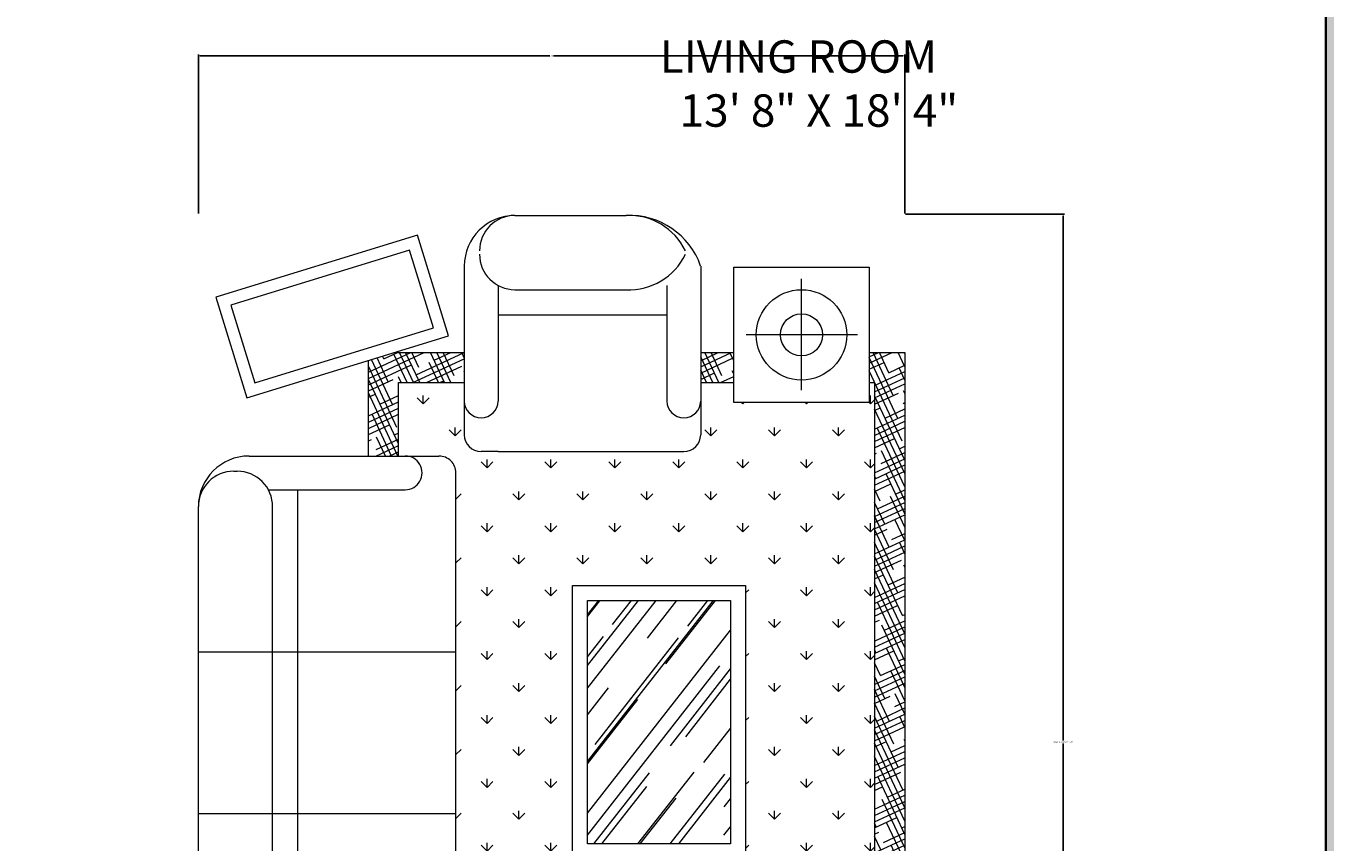
# Model space of a CAD drawing. Units: inches. Extents: x 2701 to 6846, y 811 to 2447.
# Tile 13 of 20: x 2926 to 3086, y 1130 to 1231. Entities that reach past the tile are written whole.
import ezdxf

# ---------------------------------------------------------------- set-up
doc = ezdxf.new("R2010")
doc.units = ezdxf.units.IN
for name, color, linetype, lineweight in [('A-ANNO-DIMS', 2, 'Continuous', 18), ('A-AREA-IDEN', 7, 'Continuous', 18), ('A-FURN', 8, 'Continuous', 13), ('A-WALL', 7, 'Continuous', 35)]:
    doc.layers.add(name, color=color, linetype=linetype, lineweight=lineweight)
doc.layers.add('A-WALL-PATT', color=18, linetype='Continuous', lineweight=13, true_color=0x000000)
doc.styles.get("Standard").update_dxf_attribs({"font": 'arial.ttf'})
doc.dimstyles.get("Standard").update_dxf_attribs({"dimtxt": 0.18, "dimasz": 0.18, "dimexe": 0.18, "dimexo": 0.0625, "dimgap": 0.09, "dimtad": 0, "dimtih": 1, "dimtoh": 1, "dimdec": 4, "dimzin": 0, "dimdsep": 46, "dimtxsty": 'Standard', "dimcen": 0.09, "dimadec": 0, "dimazin": 0, "dimtfac": 1, "dimtdec": 4, "dimtofl": 0, "dimtmove": 0, "dimatfit": 3, "dimfxl": 1, "dimtolj": 1, "dimtzin": 0, "dimarcsym": 0})

# ---------------------------------------------------------------- blocks, each defined once
blk = doc.blocks.new('A$C0782773B')
for p, q in [((1027.2, 2344.2), (2528, 2344.2)), ((1508.8, 2344.2), (1508.8, 1489.7)), ((2046.4, 2344.2), (2046.4, 1489.7)), ((3223.5, 2286.1), (2888.9, 2183.3)), ((3429.1, 1617), (3223.5, 2286.1)), ((909.6, 2226.6), (909.6, 2215.4)), ((2645.6, 2226.6), (2645.6, 2215.4)), ((3197, 2236.1), (2938.9, 2156.8)), ((3379.1, 1643.5), (3197, 2236.1)), ((859.2, 2176.2), (859.2, 1545.7)), ((2696, 2176.2), (2696, 1545.7)), ((2888.9, 2183.3), (3094.6, 1514.2)), ((2938.9, 2156.8), (3121.1, 1564.2)), ((971.2, 2111.9), (971.2, 1657.7)), ((1027.2, 2097.8), (2528, 2097.8)), ((2584, 2111.9), (2584, 1657.7)), ((971.2, 2013.8), (2584, 2013.8)), ((622.9, 1770.7), (643.4, 1780.2)), ((622.9, 1750), (687.8, 1780.2)), ((622.9, 1729.3), (732.1, 1780.2)), ((622.9, 1380.2), (622.9, 1780.2)), ((622.9, 1780.2), (859.2, 1780.2)), ((627.3, 1710.7), (776.5, 1780.2)), ((636.3, 1780.2), (637.5, 1777.5)), ((657, 1780.2), (686.2, 1717.5)), ((677.6, 1780.2), (724.3, 1680.2)), ((698.3, 1780.2), (745, 1680.2)), ((703.2, 1725.4), (820.8, 1780.2)), ((719, 1780.2), (765.7, 1680.2)), ((779.1, 1740.1), (859.2, 1777.4)), ((781.1, 1780.2), (788.2, 1765)), ((801.8, 1780.2), (836.9, 1705)), ((822.5, 1780.2), (859.2, 1701.5)), ((843.2, 1780.2), (859.2, 1745.8)), ((2696, 1682.3), (2906.1, 1780.2)), ((2696, 1780.2), (3012.8, 1780.2)), ((2736, 1680.2), (2950.4, 1780.2)), ((2746.5, 1780.2), (2751.2, 1770.1)), ((2767.2, 1780.2), (2799.9, 1710.1)), ((2787.9, 1780.2), (2834.5, 1680.2)), ((2790.8, 1685.1), (2994.8, 1780.2)), ((2808.5, 1780.2), (2855.2, 1680.2)), ((2829.2, 1780.2), (2875.9, 1680.2)), ((2866.7, 1699.8), (3016.1, 1769.5)), ((2891.3, 1780.2), (2901.9, 1757.6)), ((2912, 1780.2), (2950.5, 1697.6)), ((2932.7, 1780.2), (2999.2, 1637.5)), ((2953.4, 1780.2), (3039.7, 1595.1)), ((2974, 1780.2), (3039.7, 1639.5)), ((754.2, 1749.2), (786.3, 1680.2)), ((855, 1754.8), (859.2, 1756.8)), ((2696, 1703), (2835, 1767.8)), ((2696, 1755.4), (2731, 1680.2)), ((2696, 1723.7), (2759.1, 1753.1)), ((2717.2, 1754.3), (2751.7, 1680.2)), ((2867.9, 1741.8), (2896.6, 1680.2)), ((2942.6, 1714.5), (3021.7, 1751.4)), ((3018.5, 1729.2), (3027.2, 1733.3)), ((3018.5, 1729.2), (3039.7, 1683.9)), ((622.9, 1720.3), (722.9, 1505.8)), ((622.9, 1646.6), (719.1, 1691.4)), ((652.2, 1701.6), (722.9, 1550.2)), ((739.5, 1680.2), (795, 1706.1)), ((783.9, 1680.2), (859.2, 1715.4)), ((802.9, 1689.1), (807, 1680.2)), ((828.2, 1680.2), (859.2, 1694.7)), ((2696, 1711), (2710.4, 1680.2)), ((2765.9, 1694.2), (2772.4, 1680.2)), ((2939.7, 1651.1), (3034.4, 1695.3)), ((3039.7, 1692.8), (3039.7, 1461.7)), ((622.9, 1667.2), (643.2, 1676.7)), ((622.9, 1675.9), (681.6, 1549.8)), ((622.9, 1625.9), (722.9, 1672.5)), ((622.9, 1605.2), (722.9, 1651.8)), ((700.9, 1641.6), (722.9, 1594.5)), ((722.9, 1340.4), (722.9, 1680.2)), ((722.9, 1680.2), (859.2, 1680.2)), ((2696, 1680.2), (2939.7, 1680.2)), ((2916.6, 1681.7), (2917.2, 1680.2)), ((2939.7, 1671.8), (2958.5, 1680.6)), ((2939.7, 1680.2), (2939.7, 1461.7)), ((2939.7, 1630.4), (3039.7, 1677.1)), ((2939.7, 1609.7), (3039.7, 1656.4)), ((3121.1, 1564.2), (3379.1, 1643.5)), ((622.9, 1631.5), (633, 1609.9)), ((674.9, 1608.7), (722.9, 1631.1)), ((747.4, 1598.5), (767.3, 1618.4)), ((747.4, 1598.5), (775.6, 1598.5)), ((747.4, 1598.5), (767.3, 1578.6)), ((2868.8, 1598.5), (2888.7, 1618.4)), ((2868.8, 1598.5), (2896.9, 1598.5)), ((2868.8, 1598.5), (2888.7, 1578.6)), ((2939.7, 1632.1), (3019.1, 1461.7)), ((2965.3, 1621.7), (3039.7, 1462)), ((2990.2, 1612.6), (3039.7, 1635.7)), ((3094.6, 1514.2), (3429.1, 1617)), ((622.9, 1543.1), (690.7, 1574.7)), ((622.9, 1522.4), (722.9, 1569.1)), ((2939.7, 1587.7), (2994.7, 1469.9)), ((2939.7, 1547.7), (3006, 1578.6)), ((2939.7, 1527), (3039.7, 1573.6)), ((3013.9, 1561.6), (3039.7, 1506.4)), ((622.9, 1501.7), (722.9, 1548.4)), ((622.9, 1542.8), (715.9, 1343.2)), ((646.5, 1492.1), (722.9, 1527.7)), ((647.7, 1534), (722.9, 1372.7)), ((853.5, 1492.5), (871.6, 1510.6)), ((2762.7, 1492.5), (2782.6, 1512.3)), ((2939.7, 1506.3), (3039.7, 1552.9)), ((2939.7, 1543.4), (2946, 1529.9)), ((2961.8, 1495.9), (3039.7, 1532.2)), ((3037.7, 1510.6), (3039.7, 1511.5)), ((395.3, 1470.7), (915.7, 1263.8)), ((622.9, 1498.4), (677.1, 1382.2)), ((696.4, 1473.9), (722.9, 1417.1)), ((722.4, 1506.8), (722.9, 1507)), ((853.5, 1492.5), (881.6, 1492.5)), ((853.5, 1492.5), (873.4, 1472.6)), ((915.2, 1489.7), (2640, 1489.7)), ((1068.4, 1489.7), (1085.5, 1472.6)), ((1280.5, 1489.7), (1297.7, 1472.6)), ((1492.7, 1489.7), (1509.8, 1472.6)), ((1704.8, 1489.7), (1721.9, 1472.6)), ((1916.9, 1489.7), (1934.1, 1472.6)), ((2129.1, 1489.7), (2146.2, 1472.6)), ((2341.2, 1489.7), (2358.3, 1472.6)), ((2553.3, 1489.7), (2570.5, 1472.6)), ((2762.7, 1492.5), (2790.8, 1492.5)), ((2762.7, 1492.5), (2782.6, 1472.6)), ((3021.6, 1461.7), (3039.7, 1470.2)), ((622.9, 1419), (722.9, 1465.6)), ((622.9, 1439.7), (662.4, 1458.1)), ((622.9, 1454.1), (628.4, 1442.2)), ((622.9, 1398.3), (722.9, 1444.9)), ((625.9, 1379), (722.9, 1424.2)), ((3326.7, 1461.7), (2766.7, 1461.7)), ((2977.2, 1461.7), (2977.7, 1461.9)), ((694.1, 1390.1), (722.9, 1403.5)), ((747.4, 1386.4), (767.3, 1406.3)), ((747.4, 1386.4), (775.6, 1386.4)), ((747.4, 1386.4), (767.3, 1366.5)), ((959.6, 1386.4), (979.5, 1406.3)), ((959.6, 1386.4), (987.7, 1386.4)), ((959.6, 1386.4), (979.5, 1366.5)), ((1171.7, 1386.4), (1191.6, 1406.3)), ((1171.7, 1386.4), (1199.8, 1386.4)), ((1171.7, 1386.4), (1191.6, 1366.5)), ((1383.8, 1386.4), (1403.7, 1406.3)), ((1383.8, 1386.4), (1412, 1386.4)), ((1383.8, 1386.4), (1403.7, 1366.5)), ((1596, 1386.4), (1615.9, 1406.3)), ((1596, 1386.4), (1624.1, 1386.4)), ((1596, 1386.4), (1615.9, 1366.5)), ((1808.1, 1386.4), (1828, 1406.3)), ((1808.1, 1386.4), (1836.2, 1386.4)), ((1808.1, 1386.4), (1828, 1366.5)), ((2020.2, 1386.4), (2040.1, 1406.3)), ((2020.2, 1386.4), (2048.4, 1386.4)), ((2020.2, 1386.4), (2040.1, 1366.5)), ((2232.4, 1386.4), (2252.3, 1406.3)), ((2232.4, 1386.4), (2260.5, 1386.4)), ((2232.4, 1386.4), (2252.3, 1366.5)), ((2444.5, 1386.4), (2464.4, 1406.3)), ((2444.5, 1386.4), (2472.6, 1386.4)), ((2444.5, 1386.4), (2464.4, 1366.5)), ((2656.6, 1386.4), (2676.5, 1406.3)), ((2656.6, 1386.4), (2684.8, 1386.4)), ((2656.6, 1386.4), (2676.5, 1366.5)), ((2710.7, 1349.7), (2710.7, 1405.7)), ((413.6, 1342.9), (770.2, 1201.1)), ((697.7, 1350.4), (709.9, 1356.1)), ((721.7, 1340.9), (722.9, 1341.5)), ((2710.7, 1349.7), (2710.7, 733.3)), ((3262.5, 1349.7), (2878.7, 1349.7)), ((3164.3, 1349.7), (3164.3, 789.3)), ((11.5, 960), (148, 1303.4)), ((297.8, 785.9), (504.9, 1306.6)), ((859.4, 1286.2), (873.4, 1300.2)), ((1065.6, 1280.3), (1085.5, 1300.2)), ((1277.8, 1280.3), (1297.7, 1300.2)), ((1489.9, 1280.3), (1509.8, 1300.2)), ((1702, 1280.3), (1721.9, 1300.2)), ((1914.2, 1280.3), (1934.1, 1300.2)), ((2126.3, 1280.3), (2146.2, 1300.2)), ((2338.4, 1280.3), (2358.3, 1300.2)), ((2550.6, 1280.3), (2570.5, 1300.2)), ((874.1, 1280.3), (881.6, 1280.3)), ((1065.6, 1280.3), (1093.8, 1280.3)), ((1065.6, 1280.3), (1085.5, 1260.4)), ((1277.8, 1280.3), (1305.9, 1280.3)), ((1277.8, 1280.3), (1297.7, 1260.4)), ((1489.9, 1280.3), (1518, 1280.3)), ((1489.9, 1280.3), (1509.8, 1260.4)), ((1702, 1280.3), (1730.2, 1280.3)), ((1702, 1280.3), (1721.9, 1260.4)), ((1914.2, 1280.3), (1942.3, 1280.3)), ((1914.2, 1280.3), (1934.1, 1260.4)), ((2126.3, 1280.3), (2154.4, 1280.3)), ((2126.3, 1280.3), (2146.2, 1260.4)), ((2338.4, 1280.3), (2366.6, 1280.3)), ((2338.4, 1280.3), (2358.3, 1260.4)), ((2550.6, 1280.3), (2578.7, 1280.3)), ((2550.6, 1280.3), (2570.5, 1260.4)), ((3248.3, 1293.7), (3248.3, 924.1)), ((3494.7, 1293.7), (3494.7, 924.1)), ((240.4, 868.9), (377, 1212.4)), ((719.3, 618.3), (947, 1191)), ((959.6, 1174.3), (979.5, 1194.1)), ((959.6, 1174.3), (987.7, 1174.3)), ((959.6, 1174.3), (979.5, 1154.4)), ((1171.7, 1174.3), (1191.6, 1194.1)), ((1171.7, 1174.3), (1199.8, 1174.3)), ((1171.7, 1174.3), (1191.6, 1154.4)), ((1383.8, 1174.3), (1403.7, 1194.1)), ((1383.8, 1174.3), (1412, 1174.3)), ((1383.8, 1174.3), (1403.7, 1154.4)), ((1596, 1174.3), (1615.9, 1194.1)), ((1596, 1174.3), (1624.1, 1174.3)), ((1596, 1174.3), (1615.9, 1154.4)), ((1808.1, 1174.3), (1828, 1194.1)), ((1808.1, 1174.3), (1836.2, 1174.3)), ((1808.1, 1174.3), (1828, 1154.4)), ((2020.2, 1174.3), (2040.1, 1194.1)), ((2020.2, 1174.3), (2048.4, 1174.3)), ((2020.2, 1174.3), (2040.1, 1154.4)), ((2232.4, 1174.3), (2252.3, 1194.1)), ((2232.4, 1174.3), (2260.5, 1174.3)), ((2232.4, 1174.3), (2252.3, 1154.4)), ((2444.5, 1174.3), (2464.4, 1194.1)), ((2444.5, 1174.3), (2472.6, 1174.3)), ((2444.5, 1174.3), (2464.4, 1154.4)), ((2656.6, 1174.3), (2676.5, 1194.1)), ((2656.6, 1174.3), (2684.8, 1174.3)), ((2656.6, 1174.3), (2676.5, 1154.4)), ((1065.6, 1068.2), (1085.5, 1088.1)), ((1277.8, 1068.2), (1297.7, 1088.1)), ((1358.2, 528.2), (1358.2, 1102.6)), ((1358.2, 1102.6), (2266.7, 1102.6)), ((2266.7, 1102.6), (2266.7, 528.2)), ((2338.4, 1068.2), (2358.3, 1088.1)), ((2550.6, 1068.2), (2570.5, 1088.1)), ((1065.6, 1068.2), (1093.8, 1068.2)), ((1065.6, 1068.2), (1085.5, 1048.3)), ((1277.8, 1068.2), (1305.9, 1068.2)), ((1277.8, 1068.2), (1297.7, 1048.3)), ((1408.2, 578.2), (1408.2, 1052.6)), ((1408.2, 1052.6), (2216.7, 1052.6)), ((1437.7, 1052.6), (1999.3, 613.9)), ((1510.8, 1052.6), (2118.1, 578.2)), ((1674, 1052.6), (1887.9, 885.5)), ((1681.3, 1052.6), (2216.7, 634.3)), ((1837.3, 1052.6), (1926.1, 983.2)), ((1925, 1052.6), (2216.7, 824.7)), ((2000.5, 1052.6), (2216.7, 883.7)), ((2029.7, 1052.6), (2097.2, 999.9)), ((2163.7, 1052.6), (2215.4, 1012.3)), ((2168.6, 1052.6), (2216.7, 1015)), ((2216.7, 1052.6), (2216.7, 578.2)), ((2338.4, 1068.2), (2366.6, 1068.2)), ((2338.4, 1068.2), (2358.3, 1048.3)), ((2550.6, 1068.2), (2578.7, 1068.2)), ((2550.6, 1068.2), (2570.5, 1048.3)), ((1408.2, 1031.9), (1644.7, 847.1)), ((1408.2, 1005.3), (1598.7, 856.4)), ((1738, 1027.4), (2092.6, 750.4)), ((959.6, 962.1), (979.5, 982)), ((959.6, 962.1), (987.7, 962.1)), ((959.6, 962.1), (979.5, 942.2)), ((1171.7, 962.1), (1191.6, 982)), ((1171.7, 962.1), (1199.8, 962.1)), ((1171.7, 962.1), (1191.6, 942.2)), ((2136.2, 969.5), (2216.7, 906.5)), ((2444.5, 962.1), (2464.4, 982)), ((2444.5, 962.1), (2472.6, 962.1)), ((2444.5, 962.1), (2464.4, 942.2)), ((2656.6, 962.1), (2676.5, 982)), ((2656.6, 962.1), (2684.8, 962.1)), ((2656.6, 962.1), (2676.5, 942.2)), ((853.5, 856.1), (873.4, 876)), ((1065.6, 856.1), (1085.5, 876)), ((1277.8, 856.1), (1297.7, 876)), ((1408.2, 885.3), (1646.9, 698.8)), ((1408.2, 877.7), (1560.4, 758.8)), ((2338.4, 856.1), (2358.3, 876)), ((2550.6, 856.1), (2570.5, 876)), ((206.6, 822.1), (563.2, 680.3)), ((853.5, 856.1), (881.6, 856.1)), ((853.5, 856.1), (873.4, 836.2)), ((1065.6, 856.1), (1093.8, 856.1)), ((1065.6, 856.1), (1085.5, 836.2)), ((1277.8, 856.1), (1305.9, 856.1)), ((1277.8, 856.1), (1297.7, 836.2)), ((2091.6, 853.9), (2216.7, 756.2)), ((2338.4, 856.1), (2366.6, 856.1)), ((2338.4, 856.1), (2358.3, 836.2)), ((2550.6, 856.1), (2578.7, 856.1)), ((2550.6, 856.1), (2570.5, 836.2)), ((1408.2, 778.7), (1640.1, 597.6)), ((1733.4, 777.9), (1989, 578.2)), ((2006.1, 793.2), (2216.7, 628.6)), ((3262.5, 789.3), (2878.7, 789.3)), ((105.5, 741.8), (625.9, 534.9)), ((771.7, 750), (775.6, 750)), ((959.6, 750), (979.5, 769.9)), ((959.6, 750), (987.7, 750)), ((959.6, 750), (979.5, 730.1)), ((1171.7, 750), (1191.6, 769.9)), ((1171.7, 750), (1199.8, 750)), ((1171.7, 750), (1191.6, 730.1)), ((1408.2, 750.2), (1628.4, 578.2)), ((2444.5, 750), (2464.4, 769.9)), ((2444.5, 750), (2472.6, 750)), ((2444.5, 750), (2464.4, 730.1)), ((2656.6, 750), (2676.5, 769.9)), ((2656.6, 750), (2684.8, 750)), ((2656.6, 750), (2676.5, 730.1)), ((764.8, 732.7), (767.3, 730.1)), ((1764.2, 727.1), (1954.8, 578.2)), ((2131.6, 719.9), (2216.7, 653.4)), ((853.5, 643.9), (873.4, 663.8)), ((1065.6, 643.9), (1085.5, 663.8)), ((1277.8, 643.9), (1297.7, 663.8)), ((1678.6, 666.4), (1791.6, 578.2)), ((2338.4, 643.9), (2358.3, 663.8)), ((2550.6, 643.9), (2570.5, 663.8)), ((2762.7, 643.9), (2782.6, 663.8)), ((3326.7, 677.3), (2766.7, 677.3)), ((2939.7, 658.1), (2981, 677.3)), ((2939.7, 637.4), (3025.4, 677.3)), ((2939.7, 677.3), (2939.7, 567.7)), ((2939.7, 616.7), (3039.7, 663.3)), ((2950.4, 677.3), (2971.8, 631.6)), ((2971.1, 677.3), (3020.4, 571.6)), ((2991.8, 677.3), (3039.7, 574.7)), ((3012.5, 677.3), (3039.7, 619.1)), ((3039.7, 677.3), (3039.7, 567.7)), ((719.3, 618.3), (698.6, 566.2)), ((722.9, 100), (722.9, 627.2)), ((853.5, 643.9), (881.6, 643.9)), ((853.5, 643.9), (873.4, 624)), ((1065.6, 643.9), (1093.8, 643.9)), ((1065.6, 643.9), (1085.5, 624)), ((1277.8, 643.9), (1305.9, 643.9)), ((1277.8, 643.9), (1297.7, 624)), ((2338.4, 643.9), (2366.6, 643.9)), ((2338.4, 643.9), (2358.3, 624)), ((2550.6, 643.9), (2578.7, 643.9)), ((2550.6, 643.9), (2570.5, 624)), ((2762.7, 643.9), (2790.8, 643.9)), ((2762.7, 643.9), (2782.6, 624)), ((2939.7, 611.7), (2960.2, 567.7)), ((2962.7, 606.7), (3039.7, 642.6)), ((3038.6, 621.4), (3039.7, 621.9)), ((697.8, 564.3), (722.9, 576)), ((701.9, 574.6), (722.9, 529.8)), ((722.1, 575.7), (722.9, 574.1)), ((2216.7, 578.2), (1408.2, 578.2)), ((1436.7, 600.4), (1465.1, 578.2)), ((1530.9, 599.1), (1557.7, 578.2)), ((2873.3, 567.7), (3323.3, 567.7)), ((2873.3, 117.7), (2873.3, 567.7)), ((2967.7, 567.7), (2978.5, 572.7)), ((3012, 567.7), (3039.7, 580.6)), ((3323.3, 567.7), (3323.3, 117.7)), ((622.9, 508.7), (722.9, 555.3)), ((622.9, 0), (622.9, 536.1)), ((622.9, 488), (722.9, 534.6)), ((622.9, 529.4), (630.9, 533.1)), ((622.9, 522.4), (722.9, 307.9)), ((676.8, 539.8), (702.9, 483.9)), ((691.3, 553.2), (722.9, 485.4)), ((747.4, 537.9), (767.3, 557.8)), ((747.4, 537.9), (775.6, 537.9)), ((747.4, 537.9), (767.3, 518)), ((959.6, 537.9), (979.5, 557.8)), ((959.6, 537.9), (987.7, 537.9)), ((959.6, 537.9), (979.5, 518)), ((1171.7, 537.9), (1191.6, 557.8)), ((1171.7, 537.9), (1199.8, 537.9)), ((1171.7, 537.9), (1191.6, 518)), ((2266.7, 528.2), (1358.2, 528.2)), ((1393.5, 528.2), (1403.7, 518)), ((1605.7, 528.2), (1615.9, 518)), ((1817.8, 528.2), (1828, 518)), ((2029.9, 528.2), (2040.1, 518)), ((2242.1, 528.2), (2252.3, 518)), ((2444.5, 537.9), (2464.4, 557.8)), ((2444.5, 537.9), (2472.6, 537.9)), ((2444.5, 537.9), (2464.4, 518)), ((2656.6, 537.9), (2676.5, 557.8)), ((2656.6, 537.9), (2684.8, 537.9)), ((2656.6, 537.9), (2676.5, 518)), ((2868.8, 537.9), (2873.3, 542.4)), ((2868.8, 537.9), (2873.3, 537.9)), ((2868.8, 537.9), (2873.3, 533.3)), ((3098.3, 156.5), (3098.3, 526.4)), ((622.9, 478), (698.3, 316.3)), ((694.9, 500.9), (722.9, 513.9)), ((622.9, 425.9), (710.8, 466.9)), ((622.9, 446.6), (634.9, 452.2)), ((622.9, 405.3), (722.9, 451.9)), ((622.9, 433.6), (649.6, 376.3)), ((668.9, 468.1), (722.9, 352.3)), ((853.5, 431.8), (873.4, 451.7)), ((853.5, 431.8), (881.6, 431.8)), ((853.5, 431.8), (873.4, 411.9)), ((1065.6, 431.8), (1085.5, 451.7)), ((1065.6, 431.8), (1093.8, 431.8)), ((1065.6, 431.8), (1085.5, 411.9)), ((1277.8, 431.8), (1297.7, 451.7)), ((1277.8, 431.8), (1305.9, 431.8)), ((1277.8, 431.8), (1297.7, 411.9)), ((1489.9, 431.8), (1509.8, 451.7)), ((1489.9, 431.8), (1518, 431.8)), ((1489.9, 431.8), (1509.8, 411.9)), ((1702, 431.8), (1721.9, 451.7)), ((1702, 431.8), (1730.2, 431.8)), ((1702, 431.8), (1721.9, 411.9)), ((1914.2, 431.8), (1934.1, 451.7)), ((1914.2, 431.8), (1942.3, 431.8)), ((1914.2, 431.8), (1934.1, 411.9)), ((2126.3, 431.8), (2146.2, 451.7)), ((2126.3, 431.8), (2154.4, 431.8)), ((2126.3, 431.8), (2146.2, 411.9)), ((2338.4, 431.8), (2358.3, 451.7)), ((2338.4, 431.8), (2366.6, 431.8)), ((2338.4, 431.8), (2358.3, 411.9)), ((2550.6, 431.8), (2570.5, 451.7)), ((2550.6, 431.8), (2578.7, 431.8)), ((2550.6, 431.8), (2570.5, 411.9)), ((2762.7, 431.8), (2782.6, 451.7)), ((2762.7, 431.8), (2790.8, 431.8)), ((2762.7, 431.8), (2782.6, 411.9)), ((622.9, 384.6), (722.9, 431.2)), ((666.6, 384.3), (722.9, 410.5)), ((717.6, 408), (722.9, 396.7)), ((622.9, 322.5), (682.4, 350.3)), ((622.9, 301.8), (722.9, 348.4)), ((747.4, 325.7), (767.3, 345.6)), ((959.6, 325.7), (979.5, 345.6)), ((1171.7, 325.7), (1191.6, 345.6)), ((1383.8, 325.7), (1403.7, 345.6)), ((1596, 325.7), (1615.9, 345.6)), ((1808.1, 325.7), (1828, 345.6)), ((2020.2, 325.7), (2040.1, 345.6)), ((2232.4, 325.7), (2252.3, 345.6)), ((2444.5, 325.7), (2464.4, 345.6)), ((2656.6, 325.7), (2676.5, 345.6)), ((622.9, 344.9), (722.9, 130.5)), ((622.9, 281.1), (722.9, 327.8)), ((638.2, 267.6), (722.9, 307.1)), ((747.4, 325.7), (775.6, 325.7)), ((747.4, 325.7), (767.3, 305.8)), ((959.6, 325.7), (987.7, 325.7)), ((959.6, 325.7), (979.5, 305.8)), ((1171.7, 325.7), (1199.8, 325.7)), ((1171.7, 325.7), (1191.6, 305.8)), ((1383.8, 325.7), (1412, 325.7)), ((1383.8, 325.7), (1403.7, 305.8)), ((1596, 325.7), (1624.1, 325.7)), ((1596, 325.7), (1615.9, 305.8)), ((1808.1, 325.7), (1836.2, 325.7)), ((1808.1, 325.7), (1828, 305.8)), ((2020.2, 325.7), (2048.4, 325.7)), ((2020.2, 325.7), (2040.1, 305.8)), ((2232.4, 325.7), (2260.5, 325.7)), ((2232.4, 325.7), (2252.3, 305.8)), ((2444.5, 325.7), (2472.6, 325.7)), ((2444.5, 325.7), (2464.4, 305.8)), ((2656.6, 325.7), (2684.8, 325.7)), ((2656.6, 325.7), (2676.5, 305.8)), ((2868.8, 325.7), (2873.3, 330.3)), ((2868.8, 325.7), (2873.3, 325.7)), ((2868.8, 325.7), (2873.3, 321.2)), ((2914.5, 342.7), (3284.1, 342.7)), ((622.9, 300.5), (693.7, 148.6)), ((664.3, 300.4), (722.9, 174.8)), ((714.1, 282.3), (722.9, 286.4)), ((622.9, 256.2), (645, 208.7)), ((622.9, 198.4), (722.9, 245)), ((622.9, 219.1), (654.1, 233.6)), ((622.9, 177.7), (722.9, 224.3)), ((713, 240.4), (722.9, 219.2)), ((853.5, 219.7), (873.4, 239.6)), ((853.5, 219.7), (881.6, 219.7)), ((853.5, 219.7), (873.4, 199.8)), ((1065.6, 219.7), (1085.5, 239.6)), ((1065.6, 219.7), (1093.8, 219.7)), ((1065.6, 219.7), (1085.5, 199.8)), ((1277.8, 219.7), (1297.7, 239.6)), ((1277.8, 219.7), (1305.9, 219.7)), ((1277.8, 219.7), (1297.7, 199.8)), ((1489.9, 219.7), (1509.8, 239.6)), ((1489.9, 219.7), (1518, 219.7)), ((1489.9, 219.7), (1509.8, 199.8)), ((1702, 219.7), (1721.9, 239.6)), ((1702, 219.7), (1730.2, 219.7)), ((1702, 219.7), (1721.9, 199.8)), ((1914.2, 219.7), (1934.1, 239.6)), ((1914.2, 219.7), (1942.3, 219.7)), ((1914.2, 219.7), (1934.1, 199.8)), ((2126.3, 219.7), (2146.2, 239.6)), ((2126.3, 219.7), (2154.4, 219.7)), ((2126.3, 219.7), (2146.2, 199.8)), ((2338.4, 219.7), (2358.3, 239.6)), ((2338.4, 219.7), (2366.6, 219.7)), ((2338.4, 219.7), (2358.3, 199.8)), ((2550.6, 219.7), (2570.5, 239.6)), ((2550.6, 219.7), (2578.7, 219.7)), ((2550.6, 219.7), (2570.5, 199.8)), ((2762.7, 219.7), (2782.6, 239.6)), ((2762.7, 219.7), (2790.8, 219.7)), ((2762.7, 219.7), (2782.6, 199.8)), ((622.9, 157), (722.9, 203.6)), ((685.8, 165.6), (722.9, 182.9)), ((622.9, 167.4), (700.9, 0)), ((622.9, 94.9), (701.6, 131.7)), ((659.7, 132.8), (721.6, 0)), ((747.4, 113.6), (767.3, 133.5)), ((959.6, 113.6), (979.5, 133.5)), ((1171.7, 113.6), (1191.6, 133.5)), ((1383.8, 113.6), (1403.7, 133.5)), ((1596, 113.6), (1615.9, 133.5)), ((1808.1, 113.6), (1828, 133.5)), ((2020.2, 113.6), (2040.1, 133.5)), ((2232.4, 113.6), (2252.3, 133.5)), ((2444.5, 113.6), (2464.4, 133.5)), ((2656.6, 113.6), (2676.5, 133.5)), ((622.9, 123.1), (680.3, 0)), ((622.9, 74.2), (722.9, 120.9)), ((622.9, 115.6), (625.7, 116.9)), ((622.9, 53.5), (722.9, 100.2)), ((657.4, 49), (766.8, 100)), ((2939.7, 100), (722.9, 100)), ((733.3, 63.7), (811.2, 100)), ((737.1, 100), (742.4, 88.6)), ((747.4, 113.6), (775.6, 113.6)), ((747.4, 113.6), (761, 100)), ((757.8, 100), (791.1, 28.5)), ((778.4, 100), (825.1, 0)), ((799.1, 100), (845.8, 0)), ((809.2, 78.4), (855.6, 100)), ((819.8, 100), (866.5, 0)), ((863, 0), (1052.8, 88.5)), ((881.9, 100), (893, 76.1)), ((885.1, 93.1), (899.9, 100)), ((902.6, 100), (941.7, 16)), ((907.3, 0), (1121.8, 100)), ((923.3, 100), (969.9, 0)), ((943.9, 100), (990.6, 0)), ((951.7, 0), (1166.1, 100)), ((959.6, 113.6), (987.7, 113.6)), ((959.6, 113.6), (973.2, 100)), ((964.6, 100), (1011.3, 0)), ((1008.6, 5.8), (1210.5, 100)), ((1026.7, 100), (1043.7, 63.6)), ((1047.4, 100), (1092.4, 3.5)), ((1068.1, 100), (1114.7, 0)), ((1084.4, 20.5), (1254.9, 100)), ((1088.8, 100), (1135.4, 0)), ((1111.7, 95.3), (1156.1, 0)), ((1160.3, 35.2), (1299.2, 100)), ((1171.5, 100), (1194.3, 51.1)), ((1171.7, 113.6), (1199.8, 113.6)), ((1171.7, 113.6), (1185.3, 100)), ((1192.2, 100), (1238.8, 0)), ((1212.9, 100), (1259.5, 0)), ((1233.6, 100), (1280.2, 0)), ((1236.2, 49.9), (1343.6, 100)), ((1295.7, 100), (1296.3, 98.6)), ((1312.1, 64.6), (1388, 100)), ((1316.3, 100), (1345, 38.6)), ((1337, 100), (1383.7, 0)), ((1357.7, 100), (1404.3, 0)), ((1378.4, 100), (1425, 0)), ((1383.8, 113.6), (1412, 113.6)), ((1383.8, 113.6), (1397.4, 100)), ((1388, 79.3), (1432.3, 100)), ((1439.7, 0), (1631.6, 89.5)), ((1440.5, 100), (1446.9, 86.1)), ((1461.2, 100), (1495.6, 26.1)), ((1463.9, 94), (1476.7, 100)), ((1481.8, 100), (1528.5, 0)), ((1484.1, 0), (1698.5, 100)), ((1502.5, 100), (1549.2, 0)), ((1523.2, 100), (1569.9, 0)), ((1528.5, 0), (1742.9, 100)), ((1585.3, 100), (1597.6, 73.6)), ((1587.4, 6.8), (1787.3, 100)), ((1596, 113.6), (1624.1, 113.6)), ((1596, 113.6), (1609.6, 100)), ((1606, 100), (1646.3, 13.6)), ((1626.7, 100), (1673.3, 0)), ((1647.4, 100), (1694, 0)), ((1663.3, 21.5), (1831.6, 100)), ((1668, 100), (1714.7, 0)), ((1730.1, 100), (1748.2, 61.1)), ((1739.2, 36.2), (1876, 100)), ((1750.8, 100), (1796.9, 1.1)), ((1771.5, 100), (1818.1, 0)), ((1792.2, 100), (1838.8, 0)), ((1808.1, 113.6), (1836.2, 113.6)), ((1808.1, 113.6), (1821.7, 100)), ((1815.1, 50.9), (1920.4, 100)), ((1816.2, 92.8), (1859.5, 0)), ((1874.9, 100), (1898.9, 48.6)), ((1891, 65.6), (1964.7, 100)), ((1895.6, 100), (1942.2, 0)), ((1916.3, 100), (1962.9, 0)), ((1937, 100), (1983.6, 0)), ((1966.9, 80.3), (2009.1, 100)), ((1999.1, 100), (2000.8, 96.2)), ((2016.5, 0), (2210.4, 90.4)), ((2019.7, 100), (2049.5, 36.1)), ((2020.2, 113.6), (2048.4, 113.6)), ((2020.2, 113.6), (2033.8, 100)), ((2040.4, 100), (2087.1, 0)), ((2042.8, 95), (2053.5, 100)), ((2060.8, 0), (2275.3, 100)), ((2061.1, 100), (2107.8, 0)), ((2081.8, 100), (2128.4, 0)), ((2105.2, 0), (2319.7, 100)), ((2143.9, 100), (2151.5, 83.6)), ((2164.6, 100), (2200.2, 23.6)), ((2166.2, 7.8), (2364, 100)), ((2185.2, 100), (2231.9, 0)), ((2205.9, 100), (2252.6, 0)), ((2226.6, 100), (2273.3, 0)), ((2232.4, 113.6), (2260.5, 113.6)), ((2232.4, 113.6), (2246, 100)), ((2242.1, 22.5), (2408.4, 100)), ((2288.7, 100), (2302.1, 71.1)), ((2309.4, 100), (2350.8, 11.1)), ((2318, 37.2), (2452.8, 100)), ((2330.1, 100), (2376.7, 0)), ((2350.8, 100), (2397.4, 0)), ((2371.4, 100), (2418.1, 0)), ((2393.9, 51.9), (2497.1, 100)), ((2433.5, 100), (2452.8, 58.6)), ((2444.5, 113.6), (2472.6, 113.6)), ((2444.5, 113.6), (2458.1, 100)), ((2454.2, 100), (2500.8, 0)), ((2469.8, 66.6), (2541.5, 100)), ((2474.9, 100), (2521.5, 0)), ((2495.6, 100), (2542.2, 0)), ((2520.8, 90.3), (2562.9, 0)), ((2545.7, 81.3), (2585.9, 100)), ((2578.3, 100), (2603.4, 46.1)), ((2593.2, 0), (2789.2, 91.4)), ((2599, 100), (2645.6, 0)), ((2619.7, 100), (2666.3, 0)), ((2621.6, 96), (2630.2, 100)), ((2637.6, 0), (2852.1, 100)), ((2640.4, 100), (2687, 0)), ((2656.6, 113.6), (2684.8, 113.6)), ((2656.6, 113.6), (2670.2, 100)), ((2682, 0), (2896.4, 100)), ((2702.5, 100), (2705.4, 93.7)), ((2723.1, 100), (2754.1, 33.6)), ((2743.8, 100), (2790.5, 0)), ((2745, 8.7), (2978.7, 117.7)), ((2764.5, 100), (2811.2, 0)), ((2785.2, 100), (2831.8, 0)), ((2820.9, 23.4), (3023, 117.7)), ((2847.3, 100), (2856.1, 81.2)), ((2868, 100), (2904.7, 21.1)), ((2868.8, 113.6), (2873.3, 118.1)), ((2868.8, 113.6), (2896.9, 113.6)), ((2868.8, 113.6), (2882.4, 100)), ((3323.3, 117.7), (2873.3, 117.7)), ((2888.7, 100), (2935.3, 0)), ((2896.8, 38.1), (3039.7, 104.7)), ((2909.3, 100), (2956, 0)), ((2930, 100), (2976.7, 0)), ((2939.7, 117.7), (2939.7, 100)), ((2983.9, 117.7), (3006.7, 68.7)), ((3004.5, 117.7), (3039.7, 42.3)), ((3025.2, 117.7), (3039.7, 86.7)), ((3039.7, 117.7), (3039.7, 0)), ((622.9, 78.7), (640.4, 41)), ((708.4, 72.7), (742.3, 0)), ((729.9, 0), (825.1, 44.4)), ((774.2, 0), (901, 59.1)), ((818.6, 0), (976.9, 73.8)), ((859, 60.2), (887.1, 0)), ((1009.7, 47.7), (1032, 0)), ((1262.3, 82.8), (1300.9, 0)), ((1306.6, 0), (1403.9, 45.4)), ((1351, 0), (1479.8, 60.1)), ((1395.4, 0), (1555.7, 74.8)), ((1413, 70.3), (1445.7, 0)), ((1563.6, 57.8), (1590.5, 0)), ((1714.3, 45.3), (1735.4, 0)), ((1883.4, 0), (1982.7, 46.3)), ((1927.7, 0), (2058.6, 61)), ((1966.9, 80.3), (2004.3, 0)), ((1972.1, 0), (2134.5, 75.7)), ((2117.5, 67.8), (2149.1, 0)), ((2268.2, 55.3), (2293.9, 0)), ((2460.1, 0), (2561.5, 47.3)), ((2504.5, 0), (2637.4, 62)), ((2548.9, 0), (2713.3, 76.7)), ((2671.4, 77.8), (2707.7, 0)), ((2822.1, 65.3), (2852.5, 0)), ((2972.7, 52.8), (3039.7, 84.1)), ((2972.7, 52.8), (2997.3, 0)), ((641.1, 0), (673.3, 15)), ((685.5, 0), (749.2, 29.7)), ((757.1, 12.7), (763, 0)), ((907.7, 0.2), (907.8, 0)), ((1160.3, 35.2), (1176.8, 0)), ((1173.5, 0), (1176.2, 1.2)), ((1217.9, 0), (1252.1, 15.9)), ((1262.3, 0), (1328, 30.7)), ((1311, 22.7), (1321.6, 0)), ((1461.6, 10.2), (1466.4, 0)), ((1750.3, 0), (1755, 2.2)), ((1794.6, 0), (1830.9, 16.9)), ((1839, 0), (1906.8, 31.6)), ((1864.9, 32.8), (1880.2, 0)), ((2015.6, 20.3), (2025, 0)), ((2166.2, 7.8), (2169.8, 0)), ((2327, 0), (2333.8, 3.2)), ((2371.4, 0), (2409.7, 17.9)), ((2415.8, 0), (2485.6, 32.6)), ((2418.8, 42.8), (2438.8, 0)), ((2569.5, 30.3), (2583.6, 0)), ((2720.1, 17.8), (2728.4, 0)), ((2870.8, 5.3), (2873.2, 0)), ((2903.8, 0), (2912.7, 4.1)), ((2948.2, 0), (2988.6, 18.8)), ((2992.5, 0), (3039.7, 22)), ((3036.9, 0), (3039.7, 1.3)), ((3039.7, 0), (622.9, 0))]:
    blk.add_line(p, q)
for radius in [150, 70]:
    blk.add_circle((3098.3, 342.7), radius)
for centre, radius, start, end in [((1027.2, 2176.2), 168, 90, 180), ((1027.2, 2226.6), 117.6, 90, 180), ((2528, 2176.2), 168, 0, 90), ((2528, 2226.6), 117.6, 0, 90), ((1027.2, 2215.4), 117.6, 180, 270), ((2528, 2215.4), 117.6, 270, 0), ((915.2, 1657.7), 56, 180, 0), ((2640, 1657.7), 56, 180, 0), ((915.2, 1545.7), 56, 180, 270), ((2640, 1545.7), 56, 270, 0), ((384.7, 1219.9), 251, 87.5849, 160.561), ((344, 1235.6), 207.4, 93.9069, 160.9015), ((187.9, 1297.6), 207.4, 335.733, 42.7275), ((2766.7, 1405.7), 56, 90, 180), ((2878.7, 1405.7), 56, 90, 270), ((3326.7, 1293.7), 168, 0, 90), ((3365.9, 1293.7), 117.6, 90, 180), ((3377.1, 1293.7), 117.6, 0, 90), ((790.9, 1253.1), 56, 248.3172, 68.3172), ((895, 1211.7), 56, 338.3172, 68.3172), ((167.6, 897.9), 168, 158.3172, 248.3172), ((120.8, 916.5), 117.6, 158.3172, 248.3172), ((3455.5, 914.8), 207.4, 177.4158, 244.4103), ((3243.9, 914.3), 251, 289.2676, 2.2438), ((3287.6, 914.8), 207.4, 295.5897, 2.5842), ((131.2, 912.4), 117.6, 248.3172, 338.3172), ((2878.7, 733.3), 56, 90, 270), ((2766.7, 733.3), 56, 180, 270), ((542.5, 628.3), 56, 248.3172, 68.3172), ((646.6, 586.9), 56, 248.3172, 338.3172)]:
    blk.add_arc(centre, radius, start, end)
blk = doc.blocks.new('*D53')
at = {"layer": 'A-ANNO-DIMS', "color": 0, "lineweight": -2, "transparency": 16777216}
for p, q in [((3034.05, 1207.64), (3053.71, 1207.64)), ((3053.53, 1207.46), (3053.53, 1142.67)), ((3053.53, 1077.5), (3053.53, 1142.3)), ((3034.05, 1077.32), (3053.71, 1077.32))]:
    blk.add_line(p, q, dxfattribs=at)
at = {"layer": 'A-ANNO-DIMS', "color": 0, "transparency": 16777216}
for points in [[(3053.5, 1207.46), (3053.56, 1207.46), (3053.53, 1207.64)], [(3053.5, 1077.5), (3053.56, 1077.5), (3053.53, 1077.32)]]:
    blk.add_solid(points, dxfattribs=at)
at = {"layer": 'Defpoints', "color": 0, "transparency": 16777216}
for p in [(3033.98, 1207.64), (3053.53, 1207.64), (3033.98, 1077.32)]:
    blk.add_point(p, dxfattribs=at)
at = {"layer": 'A-ANNO-DIMS', "color": 0, "transparency": 16777216, "insert": (3053.53, 1142.48), "char_height": 0.18, "attachment_point": 5}
blk.add_mtext('\\A1;SEATING GROUP 130', dxfattribs=at)
blk = doc.blocks.new('*D54')
at = {"layer": 'A-ANNO-DIMS', "color": 0, "lineweight": -2, "transparency": 16777216}
for p, q in [((2946.8, 1207.71), (2946.8, 1227.37)), ((2946.98, 1227.19), (2990.17, 1227.19)), ((3033.8, 1227.19), (2990.61, 1227.19)), ((3033.98, 1207.71), (3033.98, 1227.37))]:
    blk.add_line(p, q, dxfattribs=at)
at = {"layer": 'A-ANNO-DIMS', "color": 0, "transparency": 16777216}
for points in [[(2946.98, 1227.22), (2946.98, 1227.16), (2946.8, 1227.19)], [(3033.8, 1227.22), (3033.8, 1227.16), (3033.98, 1227.19)]]:
    blk.add_solid(points, dxfattribs=at)
at = {"layer": 'Defpoints', "color": 0, "transparency": 16777216}
for p in [(2946.8, 1227.19), (2946.8, 1207.64), (3033.98, 1207.64)]:
    blk.add_point(p, dxfattribs=at)
at = {"layer": 'A-ANNO-DIMS', "color": 0, "transparency": 16777216, "insert": (2990.39, 1227.19), "char_height": 0.18, "attachment_point": 5}
blk.add_mtext('\\A1;87', dxfattribs=at)

msp = doc.modelspace()

# ---------------------------------------------------------------- hatches: boundary and pattern name
at = {"layer": 'A-WALL-PATT'}
h = msp.add_hatch(color=256, dxfattribs=at)
h.dxf.hatch_style = 1
h.paths.add_polyline_path([(3085.97, 1456.05), (3085.97, 1348.05), (3091.97, 1348.05), (3091.97, 1360.05), (3091.97, 1462.05), (2960.09, 1462.05), (2960.09, 1456.05), (2971.97, 1456.05), (2971.97, 1372.05), (2923.97, 1372.05), (2923.97, 1378.05), (2917.97, 1378.05), (2917.97, 1351.05), (2923.97, 1351.05), (2923.97, 1366.05), (2971.97, 1366.05), (2971.97, 1351.05), (2976.77, 1351.05), (2977.97, 1351.05), (2977.97, 1456.05)])
h.paths.add_polyline_path([(2779.97, 1462.05), (2779.97, 1342.05), (2785.97, 1342.05), (2785.97, 1456.05), (2917.97, 1456.05), (2917.97, 1408.05), (2922.33, 1408.05), (2923.97, 1408.05), (2923.97, 1456.05), (2937.09, 1456.05), (2937.09, 1462.05)])
h.paths.add_polyline_path([(2779.97, 1306.05), (2779.97, 1294.24), (2785.97, 1294.24), (2785.97, 1306.05), (2851.37, 1306.05, -0.025815), (2852.62, 1306.11, -0.025815), (2853.87, 1306.05), (2863.97, 1306.05), (2863.97, 1258.05), (2857.97, 1258.05), (2857.97, 1252.05), (2878.97, 1252.05), (2878.97, 1258.05), (2869.97, 1258.05), (2869.97, 1306.05), (2923.97, 1306.05), (2923.97, 1318.05), (2919.17, 1318.05), (2917.97, 1318.05), (2917.97, 1312.05), (2785.97, 1312.05), (2785.97, 1318.05), (2779.97, 1318.05)])
h.paths.add_polyline_path([(2785.97, 1252.05), (2827.97, 1252.05), (2827.97, 1256.41), (2827.97, 1258.05), (2785.97, 1258.05), (2785.97, 1271.24), (2779.97, 1271.24), (2779.97, 1174.05), (2785.97, 1174.05)])
h.paths.add_polyline_path([(2779.97, 1030.05), (2869.97, 1030.05), (2869.97, 1036.05), (2785.97, 1036.05), (2785.97, 1126.05), (2917.97, 1126.05), (2917.97, 1120.05), (2923.97, 1120.05), (2923.97, 1258.05), (2911.97, 1258.05), (2911.97, 1253.25), (2911.97, 1252.05), (2917.97, 1252.05), (2917.97, 1132.05), (2785.97, 1132.05), (2785.97, 1144.05), (2779.97, 1144.05)])
h.paths.add_polyline_path([(2935.97, 1030.05), (2935.97, 1033.05), (2935.97, 1036.05), (2923.97, 1036.05), (2923.97, 1087.05), (2919.17, 1087.05), (2917.97, 1087.05), (2917.97, 1036.05), (2893.97, 1036.05), (2893.97, 1030.05)])
h.paths.add_polyline_path([(2971.97, 1036.05), (2971.97, 1030.05), (3091.97, 1030.05), (3091.97, 1060.05), (3085.97, 1060.05), (3085.97, 1036.05)])
h.paths.add_polyline_path([(3085.97, 1084.05), (3091.97, 1084.05), (3091.97, 1096.05), (3091.97, 1268.89), (3085.97, 1268.89), (3085.97, 1258.05), (3001.97, 1258.05), (3001.97, 1270.05), (2995.97, 1270.05), (2995.97, 1252.05), (3085.97, 1252.05)])
h.paths.add_polyline_path([(3085.97, 1306.05), (3085.97, 1291.89), (3091.97, 1291.89), (3091.97, 1318.05), (3085.97, 1318.05), (3085.97, 1312.05), (2977.97, 1312.05), (2977.97, 1318.05), (2971.97, 1318.05), (2971.97, 1306.05), (2995.97, 1306.05), (2995.97, 1300.05), (3000.33, 1300.05), (3001.97, 1300.05), (3001.97, 1306.05)])

# ---------------------------------------------------------------- linework, layer by layer
at = {"layer": 'A-WALL'}
msp.add_line((3085.97, 1252.05), (3085.97, 1056.05), dxfattribs=at)

# ---------------------------------------------------------------- block references
at = {"layer": 'A-FURN', "xscale": 0.0371923082399951, "yscale": 0.0371923082399951, "zscale": 0.0371923082399951, "rotation": 90.00000000000028}
msp.add_blockref('A$C0782773B', (3033.98, 1077.51), dxfattribs=at)

# ---------------------------------------------------------------- texts
at = {"layer": 'A-AREA-IDEN', "insert": (3003.74, 1229.11), "char_height": 4, "attachment_point": 1}
msp.add_mtext_dynamic_manual_height_columns('{\\fTimes New Roman|b0|i0|c0|p18;LIVING ROOM\\P  13\' 8" X 18\' 4"}', width=44.7435, gutter_width=0, heights=[10.82], dxfattribs=at)

# ---------------------------------------------------------------- dimensions: what is measured, and where the dimension line sits
at = {"layer": 'A-ANNO-DIMS'}
dim = msp.add_linear_dim(base=(2946.8, 1227.19), p1=(3033.98, 1207.64), p2=(2946.8, 1207.64), angle=180, dimstyle='Standard', override={"dimdec": 0, "dimlfac": 1, "dimrnd": 0, "dimzin": 0, "dimdsep": 46, "dimlunit": 2}, dxfattribs=at)
dim.commit()
dim.dimension.update_dxf_attribs({"geometry": '*D54', "text_midpoint": (2990.39, 1227.19)})
dim = msp.add_linear_dim(base=(3053.53, 1207.64), p1=(3033.98, 1077.32), p2=(3033.98, 1207.64), angle=90, text='SEATING GROUP <>', dimstyle='Standard', override={"dimdec": 0, "dimlfac": 1, "dimrnd": 0, "dimzin": 0, "dimdsep": 46, "dimlunit": 2}, dxfattribs=at)
dim.commit()
dim.dimension.update_dxf_attribs({"geometry": '*D53', "text_midpoint": (3053.53, 1142.48)})

doc.saveas('drawing.dxf')
